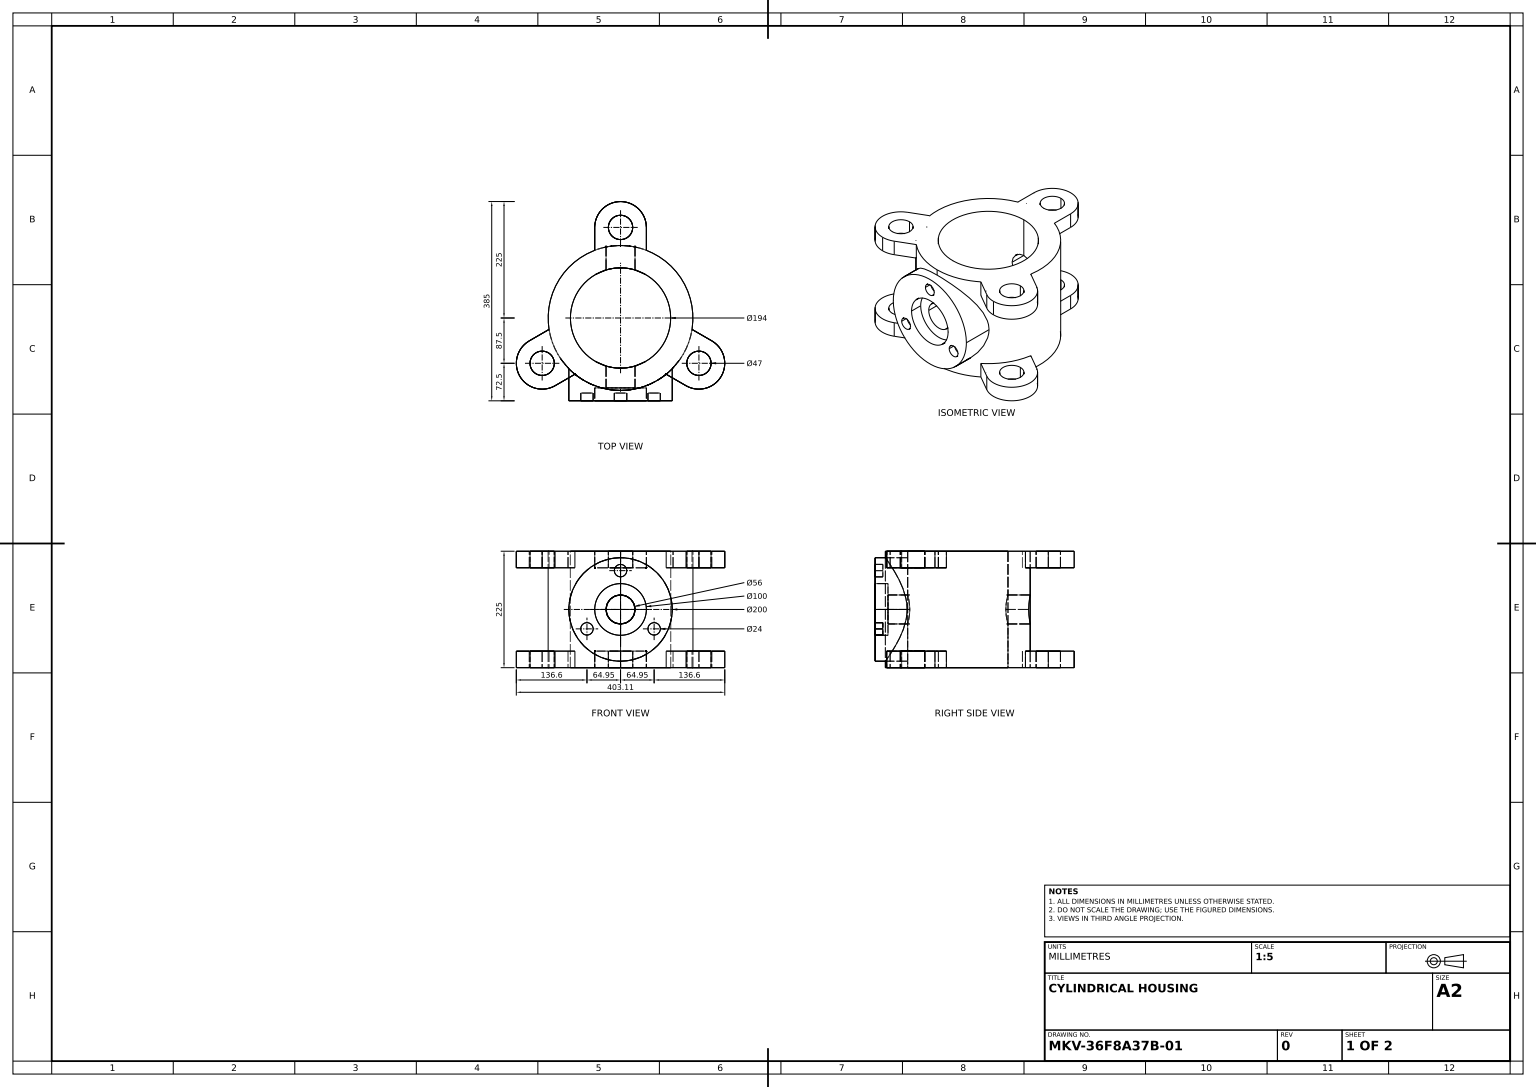
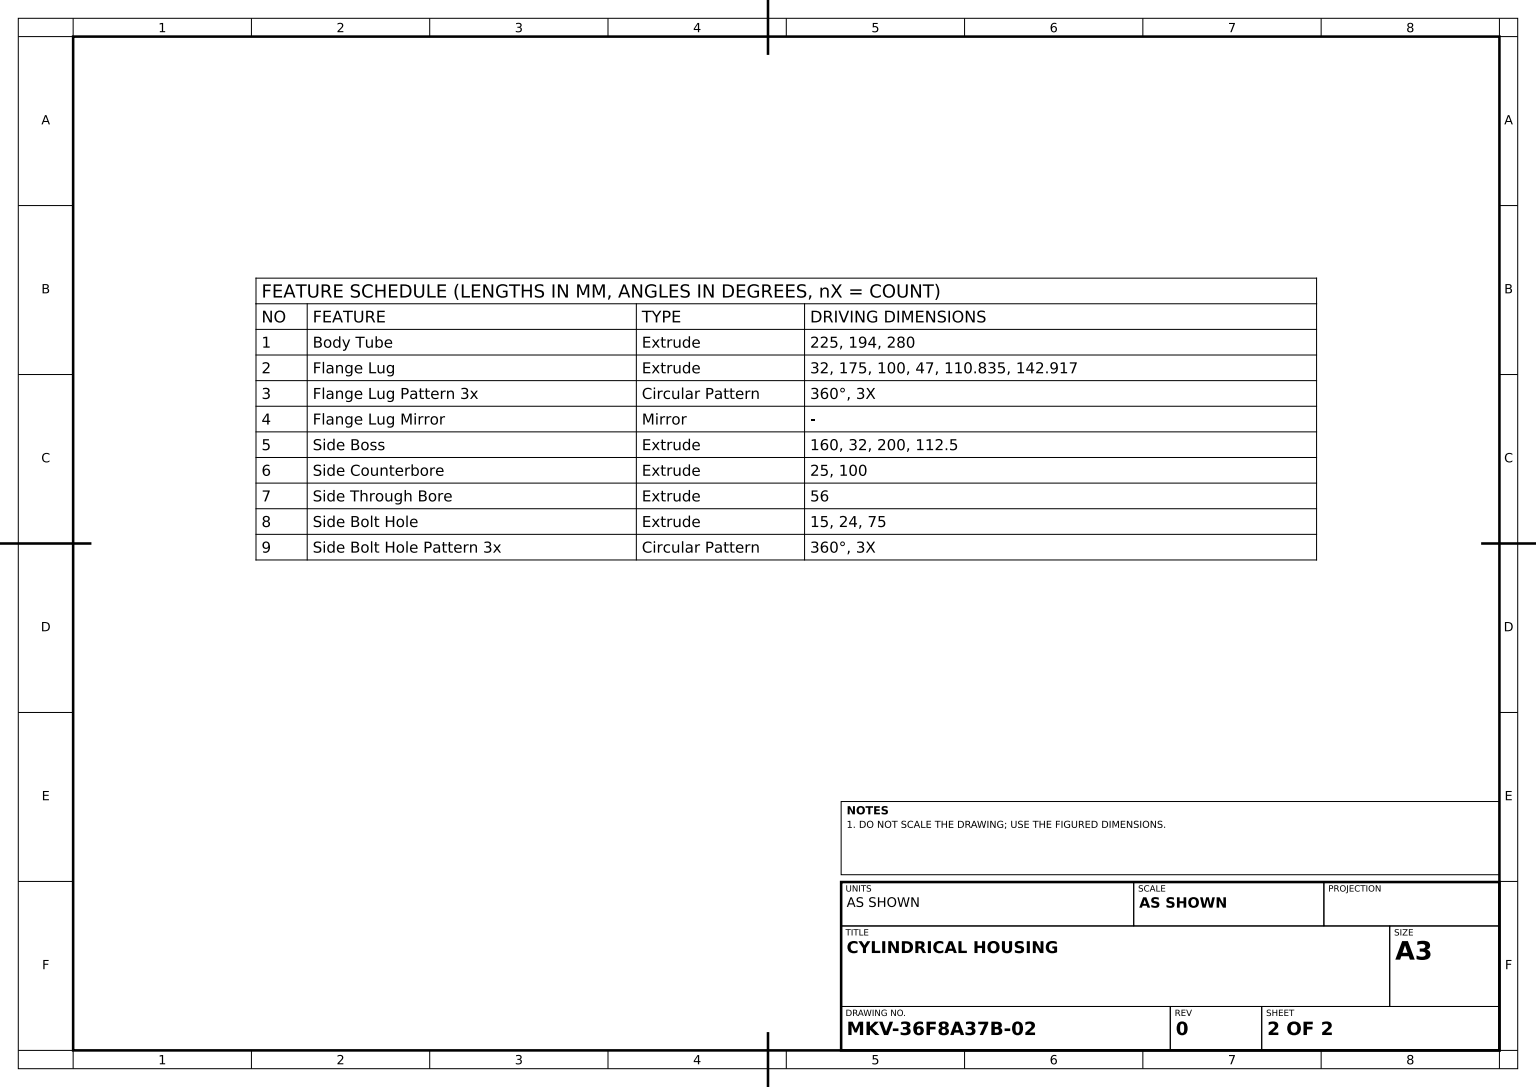
SolidWorks part; units mm, degrees
material "Plain Carbon Steel"
ref_plane "Front Plane" through (0, 0, 0) normal (0, 0, 1) x (1, 0, 0)
ref_plane "Top Plane" through (0, 0, 0) normal (0, 1, 0) x (1, 0, 0)
ref_plane "Right Plane" through (0, 0, 0) normal (1, 0, 0) x (0, 0, -1)
sketch "Body Tube Sketch" plane through (0, 0, 0) normal (0, 1, 0) x (1, 0, 0)
  circle A0 centre (0, 0) radius 140
  circle A1 centre (0, 0) radius 97
  dimension "D1" = 194
  dimension "D2" = 280
extrude "Body Tube" add sketch "Body Tube Sketch" along normal blind 225
sketch "Flange Lug Sketch" plane through (0, 225, 0) normal (0, 1, 0) x (1, 0, 0)
  line L1 (-50, 175) -> (50, 175) construction
  line L2 (-50, 175) -> (-50, 110.8347)
  line L3 (-50, 110.8347) -> (50, 110.8347)
  line L4 (50, 175) -> (50, 110.8347)
  line L5 (-50, 175) -> (50, 110.8347) construction
  line L6 (-50, 110.8347) -> (50, 175) construction
  arc A0 (50, 175) -> (-50, 175) centre (0, 175) ccw
  circle A2 centre (0, 175) radius 23.5
  circle A3 centre (0, 0) radius 140 construction
  point P0 (0, 142.9173)
  dimension "D2" = 100
  dimension "D3" = 47
  dimension "D1" = 175
  dimension "D4" = 110.8347
  dimension "D5" = 142.9173
extrude "Flange Lug" add sketch "Flange Lug Sketch" against normal blind 32
pattern_circular "Flange Lug Pattern 3x" count 3 over 360 about axis through (0, 0, 0) along (0, 1, 0) of "Flange Lug"
ref_plane "Lug Mirror Plane" through (0, 112.5, 0) normal (0, 1, 0) x (1, 0, 0)
mirror "Flange Lug Mirror" about plane through (0, 112.5, 0) normal (0, 1, 0) of "Flange Lug Pattern 3x", "Body Tube"
ref_plane "Side Boss Plane" through (0, 0, 160) normal (0, 0, 1) x (1, 0, 0)
sketch "Side Boss Sketch" plane through (0, 0, 160) normal (0, 0, 1) x (1, 0, 0)
  circle A0 centre (0, 112.5) radius 100
  dimension "D1" = 200
  dimension "D2" = 112.5
extrude "Side Boss" add sketch "Side Boss Sketch" against normal up to body
sketch "Side Counterbore Sketch" plane through (0, 0, 160) normal (0, 0, 1) x (1, 0, 0)
  circle A5 centre (0, 112.5) radius 50
  dimension "D1" = 100
extrude "Side Counterbore" cut sketch "Side Counterbore Sketch" against normal blind 25 separate body
sketch "Side Bore Sketch" plane through (0, 0, 135) normal (0, 0, 1) x (1, 0, 0)
  circle A0 centre (0, 112.5) radius 28
  dimension "D1" = 56
extrude "Side Through Bore" cut sketch "Side Bore Sketch" against normal through all
sketch "Side Bolt Hole Sketch" plane through (0, 0, 160) normal (0, 0, 1) x (1, 0, 0)
  circle A0 centre (0, 187.5) radius 12
  circle A1 centre (0, 112.5) radius 50 construction
  dimension "D1" = 24
  dimension "D2" = 75
extrude "Side Bolt Hole" cut sketch "Side Bolt Hole Sketch" against normal blind 15
pattern_circular "Side Bolt Hole Pattern 3x" count 3 over 360 about axis through (0, 112.5, 0) along (0, 0, 1) of "Side Bolt Hole"
